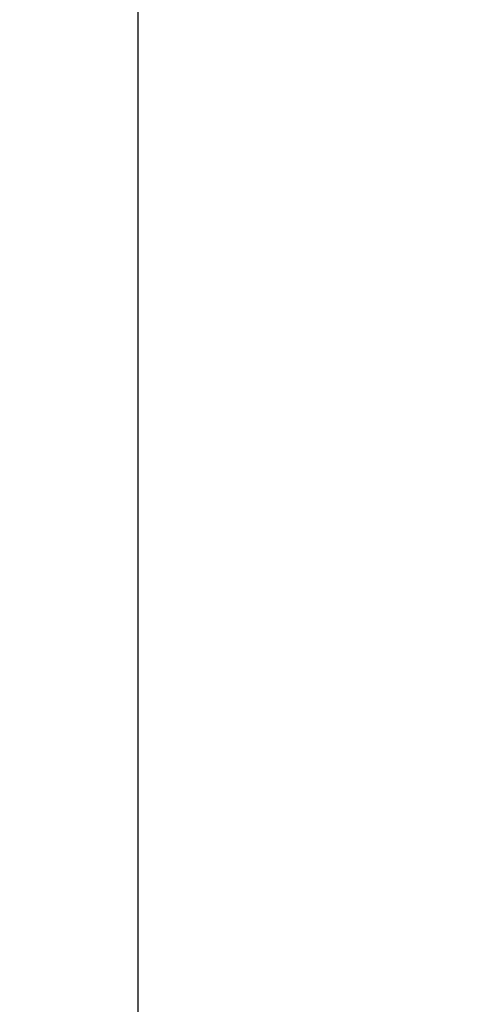
# Model space of a CAD drawing. Units: inches. Extents: x 528 to 2520, y -151 to 1354.
# Tile 3 of 41: x 542 to 587, y 1137 to 1232. Entities that reach past the tile are written whole.
import ezdxf

# ---------------------------------------------------------------- set-up
doc = ezdxf.new("R2010")
doc.units = ezdxf.units.IN
doc.header["$MEASUREMENT"] = 0
doc.layers.add('A-ANNO-DIMS', color=2, linetype='Continuous', lineweight=18)
doc.styles.get("Standard").update_dxf_attribs({"font": 'arial.ttf'})
doc.dimstyles.get("Standard").update_dxf_attribs({"dimtxt": 6, "dimasz": 2, "dimexe": 0.18, "dimexo": 0.0625, "dimgap": 0.09, "dimtad": 0, "dimtih": 1, "dimtoh": 1, "dimdec": 1, "dimzin": 0, "dimdsep": 46, "dimlunit": 3, "dimtxsty": 'Standard', "dimblk": 'ARCHTICK', "dimcen": 0.09, "dimadec": 0, "dimazin": 0, "dimtfac": 1, "dimtdec": 1, "dimtofl": 0, "dimtmove": 0, "dimatfit": 3, "dimfxl": 1, "dimtolj": 1, "dimtzin": 0, "dimarcsym": 0})

# ---------------------------------------------------------------- blocks, each defined once
blk = doc.blocks.new('_ArchTick')
at = {"color": 0, "linetype": 'ByBlock', "const_width": 0.15}
blk.add_lwpolyline([(-0.5, -0.5), (0.5, 0.5)], dxfattribs=at)
blk = doc.blocks.new('*D92')
at = {"layer": 'A-ANNO-DIMS', "color": 0, "lineweight": -2, "transparency": 16777216}
for p, q in [((586.634, 1317.103), (553.417, 1317.103)), ((553.597, 1317.103), (553.597, 1051.756)), ((553.597, 780.103), (553.597, 1045.449)), ((586.634, 780.103), (553.417, 780.103))]:
    blk.add_line(p, q, dxfattribs=at)
at = {"layer": 'Defpoints', "color": 0, "transparency": 16777216}
for p in [(553.597, 1317.103), (586.697, 1317.103), (586.697, 780.103)]:
    blk.add_point(p, dxfattribs=at)
at = {"layer": 'A-ANNO-DIMS', "color": 0, "lineweight": -2, "transparency": 16777216, "xscale": 2, "yscale": 2, "zscale": 2}
for p, rotation in [((553.597, 1317.103), 90), ((553.597, 780.103), 270)]:
    blk.add_blockref('_ArchTick', p, dxfattribs=dict(at, rotation=rotation))
at = {"layer": 'A-ANNO-DIMS', "color": 0, "transparency": 16777216, "insert": (553.597, 1048.603), "char_height": 6, "attachment_point": 5}
blk.add_mtext('\\A1;44\'-9"', dxfattribs=at)

msp = doc.modelspace()

# ---------------------------------------------------------------- dimensions: what is measured, and where the dimension line sits
at = {"layer": 'A-ANNO-DIMS'}
dim = msp.add_linear_dim(base=(553.597, 1317.103), p1=(586.697, 780.103), p2=(586.697, 1317.103), angle=90, dimstyle='Standard', override={"dimdec": 1, "dimlfac": 1, "dimrnd": 0, "dimzin": 1, "dimdsep": 46, "dimlunit": 4, "dimfrac": 2}, dxfattribs=at)
dim.commit()
dim.dimension.update_dxf_attribs({"geometry": '*D92', "text_midpoint": (553.597, 1048.603)})

doc.saveas('drawing.dxf')
